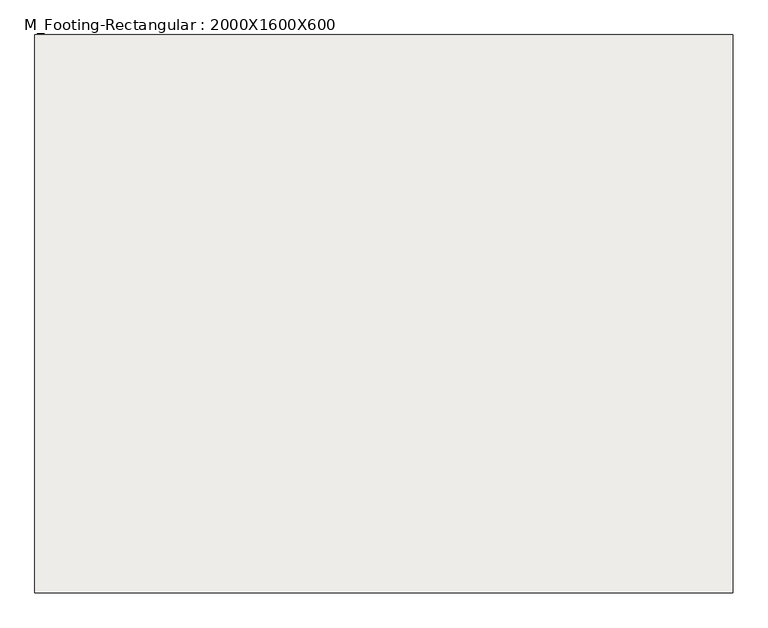
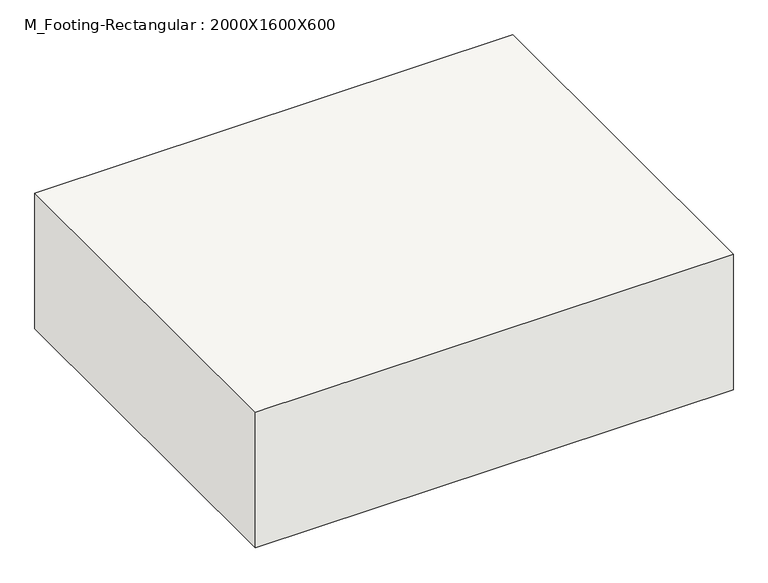
"""IFC4 building model written with IfcOpenShell, lengths in millimetres: slab geometry, M_Footing-Rectangular : 2000X1600X600."""

from ifc_helpers import new_model, si_unit, frame, origin, place, context, project, spatial, polyline, outline, extrude, source, transform, mapped, element, save


def m_footing_rectangular_2000x1600x600_a227f129(model_context):
    return source(origin(), model_context, "Body", "SweptSolid", [
        extrude(outline(polyline([(1000.0, 800.0), (1000.0, -800.0), (-1000.0, -800.0), (-1000.0, 800.0), (1000.0, 800.0)])), frame((0.0, 0.0, -600.0), z_axis=(0.0, 0.0, 1.0), x_axis=(1.0, 0.0, 0.0)), (0.0, 0.0, 1.0), 600.0),
    ])


if __name__ == "__main__":
    model = new_model("IFC4")
    model_context = context("Model", 3, world=origin())
    ifc_project = project(units=[si_unit("LENGTHUNIT", "METRE", prefix="MILLI")], contexts=[model_context])
    site = spatial("IfcSite", under=ifc_project)
    building = spatial("IfcBuilding", under=site)
    placement = place(None, origin())
    m_footing_rectangular_2000x1600x600_shape = m_footing_rectangular_2000x1600x600_a227f129(model_context)
    element("IfcSlab", 1, ObjectType="M_Footing-Rectangular : 2000X1600X600", at=placement, inside=building, context=model_context, shape_type="MappedRepresentation", body=[
        mapped(m_footing_rectangular_2000x1600x600_shape, transform((0.0, 0.0, 0.0), x_axis=(1.0, 0.0, 0.0), y_axis=(0.0, 1.0, 0.0), z_axis=(0.0, 0.0, 1.0))),
    ])
    save(model, "model.ifc")

# Revit data of these elements
# Type "M_Footing-Rectangular : 2000X1600X600"
#   Width = 2000 mm
#   Length = 1600 mm
#   Foundation Thickness = 600 mm
#   Structural Material [instance default] = Concrete, Cast-in-Place gray
#   Assembly Code = ""
# Element 1 (IfcSlab, "M_Footing-Rectangular : 2000X1600X600")
#   Structural Material = Concrete, Cast In Situ
#   Materials on its faces: "Concrete, Cast In Situ"
# Materials
#   "Concrete, Cast-in-Place gray": class "Concrete", colour RGB 192 192 192, transparency 0, Description = "Cast-in-place concrete", Cost = 0
#   "Concrete, Cast In Situ": class "Concrete", colour RGB 192 192 192, transparency 0, Description = "physical material", Cost = 0
